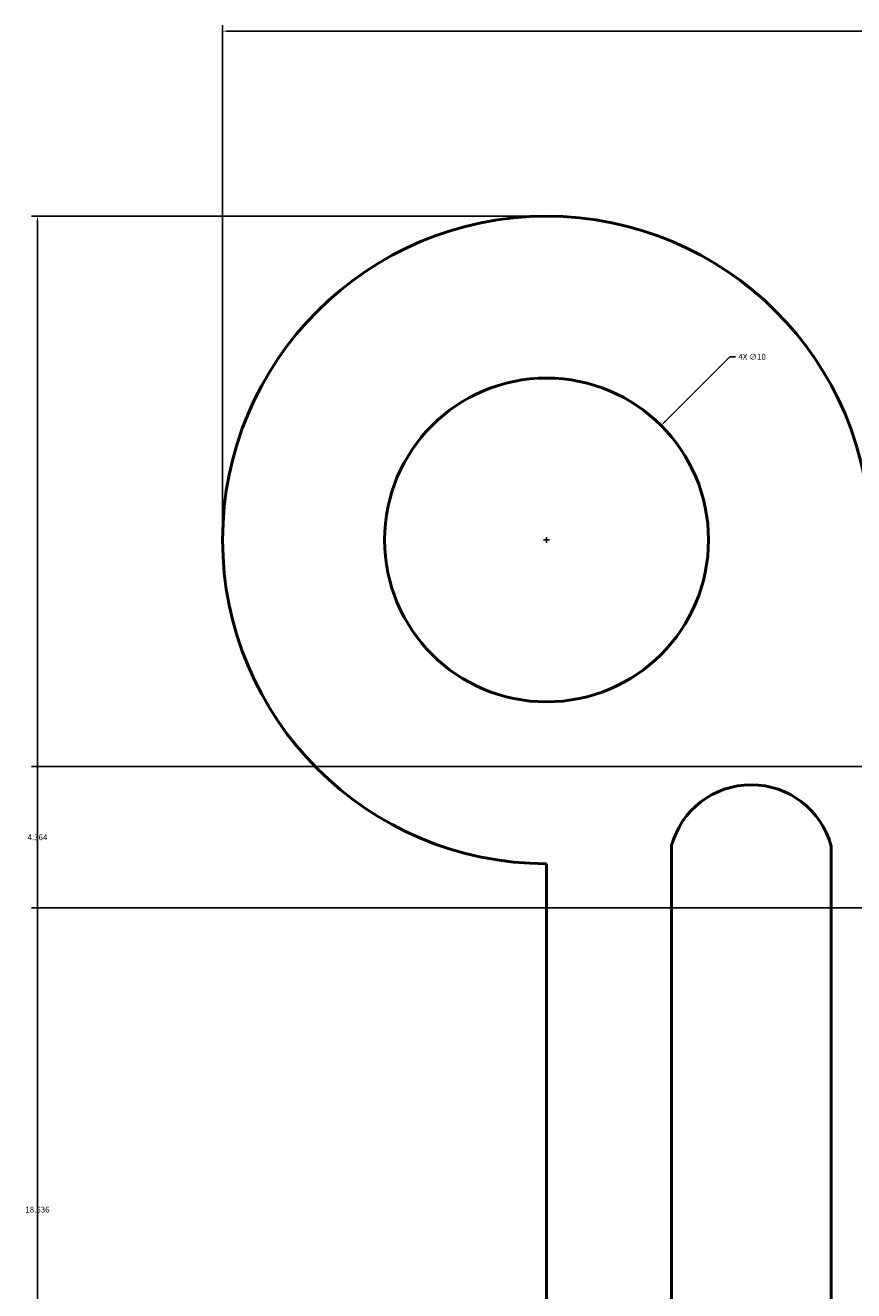
# Model space of a CAD drawing. Units: inches. Extents: x -14 to 108, y -9 to 83.
# Tile 5 of 13: x -14 to 12, y 44 to 83. Entities that reach past the tile are written whole.
import ezdxf

# ---------------------------------------------------------------- set-up
doc = ezdxf.new("R2010")
doc.units = ezdxf.units.IN
doc.header["$MEASUREMENT"] = 0
doc.layers.add('M-DIMS', color=2, linetype='Continuous', lineweight=18)
doc.layers.add('M-OUTL', color=7, linetype='Continuous', lineweight=50)
doc.styles.get("Standard").update_dxf_attribs({"font": 'arial.ttf'})
doc.dimstyles.get("Standard").update_dxf_attribs({"dimtxt": 0.18, "dimasz": 0.18, "dimexe": 0.18, "dimexo": 0.0625, "dimgap": 0.09, "dimtad": 0, "dimtih": 1, "dimtoh": 1, "dimzin": 0, "dimdsep": 46, "dimtxsty": 'Standard', "dimcen": 0.09, "dimadec": 0, "dimazin": 0, "dimtfac": 1, "dimtofl": 0, "dimtmove": 0, "dimatfit": 3, "dimfxl": 1, "dimtolj": 1, "dimtzin": 0, "dimarcsym": 0})

# ---------------------------------------------------------------- blocks, each defined once
blk = doc.blocks.new('SLOT-VERTICAL')
for points in [[(0, 1.021), (0, 40.458)], [(4.933, 40.458), (4.933, 1.021)]]:
    blk.add_lwpolyline(points)
blk.add_arc((2.466, 39.797), 2.554, 15, 165)
blk = doc.blocks.new('HOLE-D10')
blk.add_circle((5, 5), 5)
blk = doc.blocks.new('*D4')
at = {"layer": 'Defpoints', "color": 0, "transparency": 16777216}
for p in [(102.098, 82.834), (-7.902, 67.119), (102.098, 67.119)]:
    blk.add_point(p, dxfattribs=at)
at = {"layer": 'M-DIMS', "color": 0, "lineweight": -2, "transparency": 16777216}
for p, q in [((-7.902, 67.182), (-7.902, 83.014)), ((102.098, 67.182), (102.098, 83.014)), ((-7.722, 82.834), (46.818, 82.834)), ((101.918, 82.834), (47.378, 82.834))]:
    blk.add_line(p, q, dxfattribs=at)
at = {"layer": 'M-DIMS', "color": 0, "transparency": 16777216}
for points in [[(-7.722, 82.864), (-7.722, 82.804), (-7.902, 82.834)], [(101.918, 82.864), (101.918, 82.804), (102.098, 82.834)]]:
    blk.add_solid(points, dxfattribs=at)
at = {"layer": 'M-DIMS', "color": 0, "transparency": 16777216, "insert": (47.098, 82.834), "char_height": 0.18, "attachment_point": 5}
blk.add_mtext('\\A1;110', dxfattribs=at)
blk = doc.blocks.new('*D5')
at = {"layer": 'Defpoints', "color": 0, "transparency": 16777216}
for p in [(-13.617, 77.119), (2.098, 77.119), (2.098, -2.881)]:
    blk.add_point(p, dxfattribs=at)
at = {"layer": 'M-DIMS', "color": 0, "lineweight": -2, "transparency": 16777216}
for p, q in [((2.035, 77.119), (-13.797, 77.119)), ((-13.617, 76.939), (-13.617, 37.301)), ((-13.617, -2.701), (-13.617, 36.937)), ((2.035, -2.881), (-13.797, -2.881))]:
    blk.add_line(p, q, dxfattribs=at)
at = {"layer": 'M-DIMS', "color": 0, "transparency": 16777216}
for points in [[(-13.647, 76.939), (-13.587, 76.939), (-13.617, 77.119)], [(-13.647, -2.701), (-13.587, -2.701), (-13.617, -2.881)]]:
    blk.add_solid(points, dxfattribs=at)
at = {"layer": 'M-DIMS', "color": 0, "transparency": 16777216, "insert": (-13.617, 37.119), "char_height": 0.18, "attachment_point": 5}
blk.add_mtext('\\A1;80', dxfattribs=at)
blk = doc.blocks.new('*D18')
at = {"layer": 'Defpoints', "color": 0, "transparency": 16777216}
for p in [(-13.617, 55.756), (26.462, 55.756), (16.928, 37.119)]:
    blk.add_point(p, dxfattribs=at)
at = {"layer": 'M-DIMS', "color": 0, "lineweight": -2, "transparency": 16777216}
for p, q in [((26.399, 55.756), (-13.797, 55.756)), ((-13.617, 55.576), (-13.617, 46.619)), ((-13.617, 37.299), (-13.617, 46.256)), ((16.865, 37.119), (-13.797, 37.119))]:
    blk.add_line(p, q, dxfattribs=at)
at = {"layer": 'M-DIMS', "color": 0, "transparency": 16777216}
for points in [[(-13.647, 55.576), (-13.587, 55.576), (-13.617, 55.756)], [(-13.647, 37.299), (-13.587, 37.299), (-13.617, 37.119)]]:
    blk.add_solid(points, dxfattribs=at)
at = {"layer": 'M-DIMS', "color": 0, "transparency": 16777216, "insert": (-13.617, 46.437), "char_height": 0.18, "attachment_point": 5}
blk.add_mtext('\\A1;18.636', dxfattribs=at)
blk = doc.blocks.new('*D23')
at = {"layer": 'Defpoints', "color": 0, "transparency": 16777216}
for p in [(-13.617, 60.119), (47.098, 60.119), (26.462, 55.756)]:
    blk.add_point(p, dxfattribs=at)
at = {"layer": 'M-DIMS', "color": 0, "lineweight": -2, "transparency": 16777216}
for p, q in [((47.035, 60.119), (-13.797, 60.119)), ((-13.617, 59.939), (-13.617, 58.119)), ((-13.617, 55.936), (-13.617, 57.756)), ((26.399, 55.756), (-13.797, 55.756))]:
    blk.add_line(p, q, dxfattribs=at)
at = {"layer": 'M-DIMS', "color": 0, "transparency": 16777216}
for points in [[(-13.647, 59.939), (-13.587, 59.939), (-13.617, 60.119)], [(-13.647, 55.936), (-13.587, 55.936), (-13.617, 55.756)]]:
    blk.add_solid(points, dxfattribs=at)
at = {"layer": 'M-DIMS', "color": 0, "transparency": 16777216, "insert": (-13.617, 57.937), "char_height": 0.18, "attachment_point": 5}
blk.add_mtext('\\A1;4.364', dxfattribs=at)
blk = doc.blocks.new('*D25')
at = {"layer": 'Defpoints', "color": 0, "transparency": 16777216}
for p in [(5.634, 70.655), (-1.438, 63.584)]:
    blk.add_point(p, dxfattribs=at)
at = {"layer": 'M-DIMS', "color": 0, "lineweight": -2, "transparency": 16777216}
for p, q in [((7.755, 72.776), (5.761, 70.782)), ((7.935, 72.776), (7.755, 72.776)), ((2.008, 67.119), (2.188, 67.119)), ((2.098, 67.029), (2.098, 67.209))]:
    blk.add_line(p, q, dxfattribs=at)
at = {"layer": 'M-DIMS', "color": 0, "transparency": 16777216}
blk.add_solid([(5.74, 70.803), (5.782, 70.761), (5.634, 70.655)], dxfattribs=at)
at = {"layer": 'M-DIMS', "color": 0, "transparency": 16777216, "insert": (8.444, 72.776), "char_height": 0.18, "attachment_point": 5}
blk.add_mtext('\\A1;4X ∅10', dxfattribs=at)

msp = doc.modelspace()

# ---------------------------------------------------------------- linework, layer by layer
at = {"layer": 'M-OUTL'}
msp.add_lwpolyline([(2.0979, 57.1193), (2.0979, 17.1193)], dxfattribs=at)
msp.add_arc((2.0979, 67.1193), 10, 0, 270, dxfattribs=at)

# ---------------------------------------------------------------- block references
for name, p in [('HOLE-D10', (-2.902, 62.119)), ('HOLE-D10', (-2.902, 62.119)), ('SLOT-VERTICAL', (5.9511, 17.206))]:
    msp.add_blockref(name, p, dxfattribs=at)

# ---------------------------------------------------------------- dimensions: what is measured, and where the dimension line sits
at = {"layer": 'M-DIMS'}
dim = msp.add_linear_dim(base=(102.0979, 82.8343), p1=(-7.9021, 67.1193), p2=(102.0979, 67.1193), dimstyle='Standard', override={"dimdec": 0, "dimlfac": 1, "dimrnd": 0, "dimzin": 0, "dimdsep": 46, "dimlunit": 2}, dxfattribs=at)
dim.commit()
dim.dimension.update_dxf_attribs({"geometry": '*D4', "text_midpoint": (47.0979, 82.8343)})
for base, p1, p2, override, picture, middle in [((-13.6171, 77.1193), (2.0979, -2.8807), (2.0979, 77.1193), {"dimdec": 0, "dimlfac": 1, "dimrnd": 0, "dimzin": 0, "dimdsep": 46, "dimlunit": 2}, '*D5', (-13.6171, 37.1193)), ((-13.6171, 60.1193), (26.4616, 55.7556), (47.0979, 60.1193), {"dimdec": 3, "dimlfac": 1, "dimrnd": 0, "dimzin": 0, "dimdsep": 46, "dimlunit": 2}, '*D23', (-13.6171, 57.9375)), ((-13.6171, 55.7556), (16.9278, 37.1193), (26.4616, 55.7556), {"dimdec": 3, "dimlfac": 1, "dimrnd": 0, "dimzin": 0, "dimdsep": 46, "dimlunit": 2}, '*D18', (-13.6171, 46.4375))]:
    dim = msp.add_linear_dim(base=base, p1=p1, p2=p2, angle=90, dimstyle='Standard', override=override, dxfattribs=at)
    dim.commit()
    dim.dimension.update_dxf_attribs({"geometry": picture, "text_midpoint": middle})
dim = msp.add_diameter_dim_2p(p1=(-1.4378, 63.584), p2=(5.6337, 70.6547), text='4X <>', dimstyle='Standard', override={"dimdec": 0, "dimlfac": 1, "dimrnd": 0, "dimzin": 0, "dimdsep": 46, "dimlunit": 2}, dxfattribs=at)
dim.commit()
dim.dimension.update_dxf_attribs({"geometry": '*D25', "text_midpoint": (8.4439, 72.7759), "dimtype": 163})

doc.saveas('drawing.dxf')
